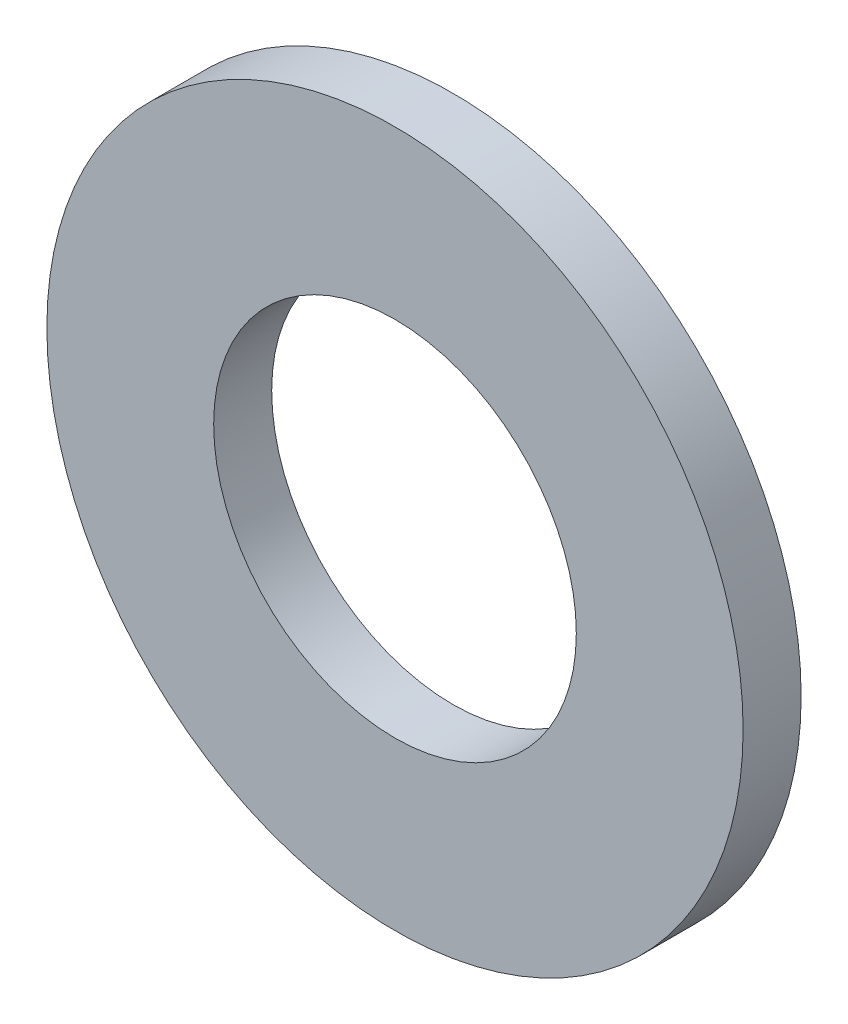
ISO-10303-21;
HEADER;
FILE_DESCRIPTION(('STEP AP214'),'2;1');
FILE_NAME('part.step','',(''),(''),'','','');
FILE_SCHEMA(('AUTOMOTIVE_DESIGN { 1 0 10303 214 1 1 1 1 }'));
ENDSEC;
DATA;
#1=APPLICATION_CONTEXT('core data for automotive mechanical design processes');
#2=APPLICATION_PROTOCOL_DEFINITION('international standard','automotive_design',2000,#1);
#3=PRODUCT_CONTEXT('',#1,'mechanical');
#4=PRODUCT('Part','Part','',(#3));
#5=PRODUCT_RELATED_PRODUCT_CATEGORY('part','',(#4));
#6=PRODUCT_DEFINITION_FORMATION('','',#4);
#7=PRODUCT_DEFINITION_CONTEXT('part definition',#1,'design');
#8=PRODUCT_DEFINITION('design','',#6,#7);
#9=PRODUCT_DEFINITION_SHAPE('','',#8);
#10=(LENGTH_UNIT() NAMED_UNIT(*) SI_UNIT(.MILLI.,.METRE.));
#11=(NAMED_UNIT(*) PLANE_ANGLE_UNIT() SI_UNIT($,.RADIAN.));
#12=(NAMED_UNIT(*) SI_UNIT($,.STERADIAN.) SOLID_ANGLE_UNIT());
#13=UNCERTAINTY_MEASURE_WITH_UNIT(LENGTH_MEASURE(1.E-05),#10,'distance_accuracy_value','');
#14=(GEOMETRIC_REPRESENTATION_CONTEXT(3) GLOBAL_UNCERTAINTY_ASSIGNED_CONTEXT((#13)) GLOBAL_UNIT_ASSIGNED_CONTEXT((#10,
#11,#12)) REPRESENTATION_CONTEXT('',''));
#15=CARTESIAN_POINT('',(0.,0.,0.));
#16=DIRECTION('',(0.,0.,1.));
#17=DIRECTION('',(1.,0.,0.));
#18=AXIS2_PLACEMENT_3D('',#15,#16,#17);
#19=CARTESIAN_POINT('',(0.,0.,0.5));
#20=DIRECTION('',(0.,0.,1.));
#21=DIRECTION('',(1.,0.,0.));
#22=AXIS2_PLACEMENT_3D('',#19,#20,#21);
#23=PLANE('',#22);
#24=CARTESIAN_POINT('',(0.,0.,0.5));
#25=DIRECTION('',(0.,0.,1.));
#26=DIRECTION('',(1.,0.,0.));
#27=AXIS2_PLACEMENT_3D('',#24,#25,#26);
#28=CIRCLE('',#27,6.);
#29=CARTESIAN_POINT('',(6.,0.,0.5));
#30=VERTEX_POINT('',#29);
#31=EDGE_CURVE('E10',#30,#30,#28,.T.);
#32=ORIENTED_EDGE('',*,*,#31,.T.);
#33=EDGE_LOOP('',(#32));
#34=FACE_BOUND('',#33,.T.);
#35=CARTESIAN_POINT('',(0.,0.,0.5));
#36=DIRECTION('',(0.,0.,1.));
#37=DIRECTION('',(1.,0.,0.));
#38=AXIS2_PLACEMENT_3D('',#35,#36,#37);
#39=CIRCLE('',#38,3.125);
#40=CARTESIAN_POINT('',(3.125,0.,0.5));
#41=VERTEX_POINT('',#40);
#42=EDGE_CURVE('E55',#41,#41,#39,.T.);
#43=ORIENTED_EDGE('',*,*,#42,.F.);
#44=EDGE_LOOP('',(#43));
#45=FACE_BOUND('',#44,.T.);
#46=ADVANCED_FACE('F41',(#34,#45),#23,.T.);
#47=CARTESIAN_POINT('',(0.,0.,-0.5));
#48=DIRECTION('',(0.,0.,1.));
#49=DIRECTION('',(1.,0.,0.));
#50=AXIS2_PLACEMENT_3D('',#47,#48,#49);
#51=PLANE('',#50);
#52=CARTESIAN_POINT('',(0.,0.,-0.5));
#53=DIRECTION('',(0.,0.,1.));
#54=DIRECTION('',(1.,0.,0.));
#55=AXIS2_PLACEMENT_3D('',#52,#53,#54);
#56=CIRCLE('',#55,6.);
#57=CARTESIAN_POINT('',(6.,0.,-0.5));
#58=VERTEX_POINT('',#57);
#59=EDGE_CURVE('E44',#58,#58,#56,.T.);
#60=ORIENTED_EDGE('',*,*,#59,.F.);
#61=EDGE_LOOP('',(#60));
#62=FACE_BOUND('',#61,.T.);
#63=CARTESIAN_POINT('',(0.,0.,-0.5));
#64=DIRECTION('',(0.,0.,1.));
#65=DIRECTION('',(1.,0.,0.));
#66=AXIS2_PLACEMENT_3D('',#63,#64,#65);
#67=CIRCLE('',#66,3.125);
#68=CARTESIAN_POINT('',(3.125,0.,-0.5));
#69=VERTEX_POINT('',#68);
#70=EDGE_CURVE('E53',#69,#69,#67,.T.);
#71=ORIENTED_EDGE('',*,*,#70,.T.);
#72=EDGE_LOOP('',(#71));
#73=FACE_BOUND('',#72,.T.);
#74=ADVANCED_FACE('F61',(#62,#73),#51,.F.);
#75=CARTESIAN_POINT('',(0.,0.,0.5));
#76=DIRECTION('',(0.,0.,-1.));
#77=DIRECTION('',(-1.,0.,0.));
#78=AXIS2_PLACEMENT_3D('',#75,#76,#77);
#79=CYLINDRICAL_SURFACE('',#78,6.);
#80=ORIENTED_EDGE('',*,*,#31,.F.);
#81=EDGE_LOOP('',(#80));
#82=FACE_BOUND('',#81,.T.);
#83=ORIENTED_EDGE('',*,*,#59,.T.);
#84=EDGE_LOOP('',(#83));
#85=FACE_BOUND('',#84,.T.);
#86=ADVANCED_FACE('F43',(#82,#85),#79,.T.);
#87=CARTESIAN_POINT('',(0.,0.,0.5));
#88=DIRECTION('',(0.,0.,-1.));
#89=DIRECTION('',(-1.,0.,0.));
#90=AXIS2_PLACEMENT_3D('',#87,#88,#89);
#91=CYLINDRICAL_SURFACE('',#90,3.125);
#92=ORIENTED_EDGE('',*,*,#42,.T.);
#93=EDGE_LOOP('',(#92));
#94=FACE_BOUND('',#93,.T.);
#95=ORIENTED_EDGE('',*,*,#70,.F.);
#96=EDGE_LOOP('',(#95));
#97=FACE_BOUND('',#96,.T.);
#98=ADVANCED_FACE('F58',(#94,#97),#91,.F.);
#99=CLOSED_SHELL('',(#46,#74,#86,#98));
#100=MANIFOLD_SOLID_BREP('B2',#99);
#101=ADVANCED_BREP_SHAPE_REPRESENTATION('',(#18,#100),#14);
#102=SHAPE_DEFINITION_REPRESENTATION(#9,#101);
ENDSEC;
END-ISO-10303-21;
